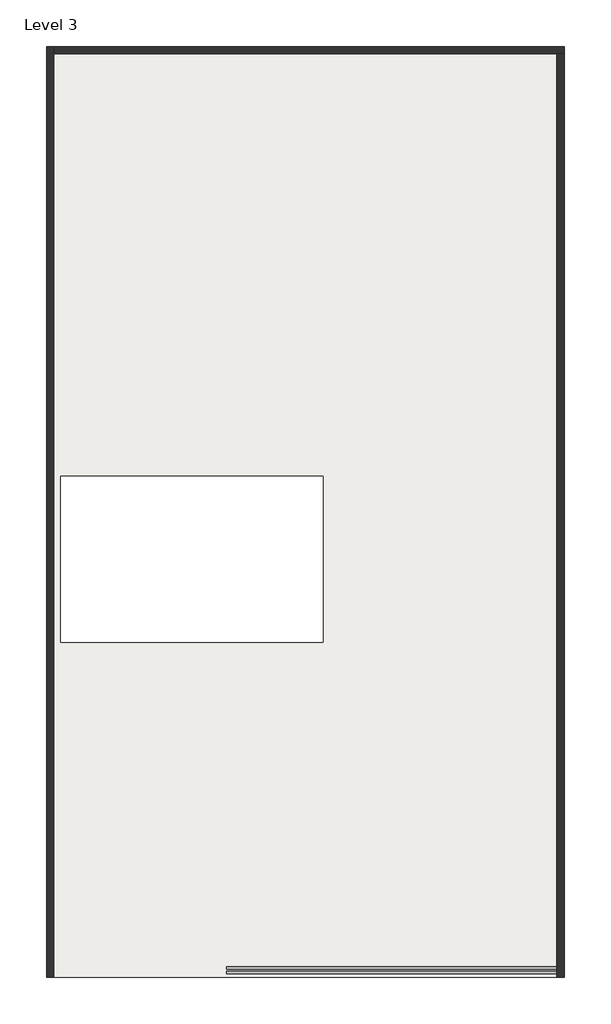
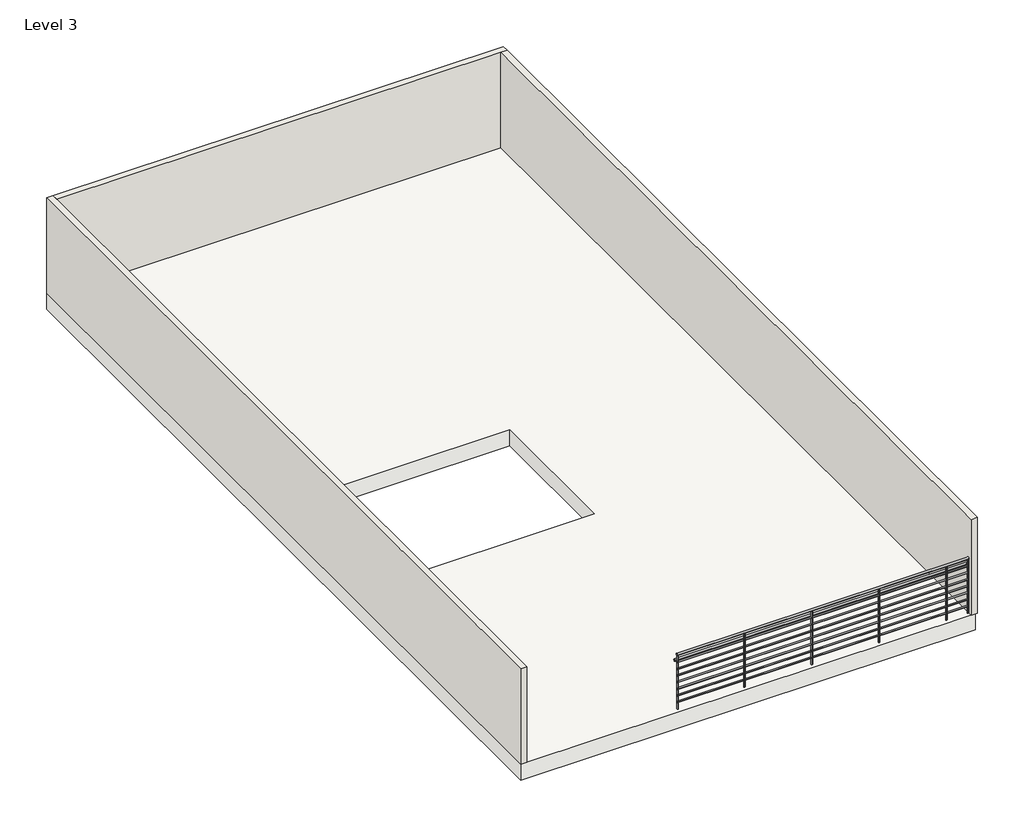
# One storey: 3 walls, 1 railing, 1 slab.
"""IFC4 building model written with IfcOpenShell, lengths in millimetres."""

from ifc_helpers import new_model, si_unit, point, frame, frame_2d, origin, place, context, project, spatial, polyline, circle_curve, trimmed, segment, composite_curve, outline, extrude, faceted_brep, element, save

model = new_model("IFC4")

# Units and contexts
model_context = context("Model", 3, world=origin())
ifc_project = project(units=[si_unit("LENGTHUNIT", "METRE", prefix="MILLI")], contexts=[model_context])

# Site, building, storey
site = spatial("IfcSite", under=ifc_project)
building = spatial("IfcBuilding", under=site)
storey = spatial("IfcBuildingStorey", under=building, Name="Level 3", Elevation=6400.8)

# Railing
placement = place(None, origin())
element("IfcRailing", 1, ObjectType="Guardrail - Pipe", at=placement, inside=storey, context=model_context, shape_type="SweptSolid", body=[
    extrude(outline(composite_curve([segment(trimmed(circle_curve(frame_2d((-4166.2834906, 7296.15)), 19.05), [point((-4185.3334906, 7296.15))], [point((-4147.2334906, 7296.15))], False, "CARTESIAN"), True, "CONTINUOUS"), segment(trimmed(circle_curve(frame_2d((-4166.2834906, 7296.15)), 19.05), [point((-4147.2334906, 7296.15))], [point((-4185.3334906, 7296.15))], False, "CARTESIAN"), True, "CONTINUOUS")], self_intersect=False)), frame((-11047.3280281, 0.0, 0.0), z_axis=(1.0, 0.0, 0.0), x_axis=(0.0, 1.0, 0.0)), (0.0, 0.0, 1.0), 5278.8112572),
    extrude(outline(composite_curve([segment(trimmed(circle_curve(frame_2d((-4242.4834906, 7448.55)), 19.05), [point((-4261.5334906, 7448.55))], [point((-4223.4334906, 7448.55))], False, "CARTESIAN"), True, "CONTINUOUS"), segment(trimmed(circle_curve(frame_2d((-4242.4834906, 7448.55)), 19.05), [point((-4223.4334906, 7448.55))], [point((-4261.5334906, 7448.55))], False, "CARTESIAN"), True, "CONTINUOUS")], self_intersect=False)), frame((-11047.3280281, 0.0, 0.0), z_axis=(1.0, 0.0, 0.0), x_axis=(0.0, 1.0, 0.0)), (0.0, 0.0, 1.0), 5278.8112572),
    extrude(outline(composite_curve([segment(trimmed(circle_curve(frame_2d((-4242.4834906, 7302.5)), 12.7), [point((-4229.7834906, 7302.5))], [point((-4255.1834906, 7302.5))], False, "CARTESIAN"), True, "CONTINUOUS"), segment(trimmed(circle_curve(frame_2d((-4242.4834906, 7302.5)), 12.7), [point((-4255.1834906, 7302.5))], [point((-4229.7834906, 7302.5))], False, "CARTESIAN"), True, "CONTINUOUS")], self_intersect=False)), frame((-11047.3280281, 0.0, 0.0), z_axis=(1.0, 0.0, 0.0), x_axis=(0.0, 1.0, 0.0)), (0.0, 0.0, 1.0), 5278.8112572),
    extrude(outline(composite_curve([segment(trimmed(circle_curve(frame_2d((-4242.4834906, 7175.5)), 12.7), [point((-4229.7834906, 7175.5))], [point((-4255.1834906, 7175.5))], False, "CARTESIAN"), True, "CONTINUOUS"), segment(trimmed(circle_curve(frame_2d((-4242.4834906, 7175.5)), 12.7), [point((-4255.1834906, 7175.5))], [point((-4229.7834906, 7175.5))], False, "CARTESIAN"), True, "CONTINUOUS")], self_intersect=False)), frame((-11047.3280281, 0.0, 0.0), z_axis=(1.0, 0.0, 0.0), x_axis=(0.0, 1.0, 0.0)), (0.0, 0.0, 1.0), 5278.8112572),
    extrude(outline(composite_curve([segment(trimmed(circle_curve(frame_2d((-4242.4834906, 7048.5)), 12.7), [point((-4229.7834906, 7048.5))], [point((-4255.1834906, 7048.5))], False, "CARTESIAN"), True, "CONTINUOUS"), segment(trimmed(circle_curve(frame_2d((-4242.4834906, 7048.5)), 12.7), [point((-4255.1834906, 7048.5))], [point((-4229.7834906, 7048.5))], False, "CARTESIAN"), True, "CONTINUOUS")], self_intersect=False)), frame((-11047.3280281, 0.0, 0.0), z_axis=(1.0, 0.0, 0.0), x_axis=(0.0, 1.0, 0.0)), (0.0, 0.0, 1.0), 5278.8112572),
    extrude(outline(composite_curve([segment(trimmed(circle_curve(frame_2d((-4242.4834906, 6921.5)), 12.7), [point((-4229.7834906, 6921.5))], [point((-4255.1834906, 6921.5))], False, "CARTESIAN"), True, "CONTINUOUS"), segment(trimmed(circle_curve(frame_2d((-4242.4834906, 6921.5)), 12.7), [point((-4255.1834906, 6921.5))], [point((-4229.7834906, 6921.5))], False, "CARTESIAN"), True, "CONTINUOUS")], self_intersect=False)), frame((-11047.3280281, 0.0, 0.0), z_axis=(1.0, 0.0, 0.0), x_axis=(0.0, 1.0, 0.0)), (0.0, 0.0, 1.0), 5278.8112572),
    extrude(outline(composite_curve([segment(trimmed(circle_curve(frame_2d((-4242.4834906, 6794.5)), 12.7), [point((-4229.7834906, 6794.5))], [point((-4255.1834906, 6794.5))], False, "CARTESIAN"), True, "CONTINUOUS"), segment(trimmed(circle_curve(frame_2d((-4242.4834906, 6794.5)), 12.7), [point((-4255.1834906, 6794.5))], [point((-4229.7834906, 6794.5))], False, "CARTESIAN"), True, "CONTINUOUS")], self_intersect=False)), frame((-11047.3280281, 0.0, 0.0), z_axis=(1.0, 0.0, 0.0), x_axis=(0.0, 1.0, 0.0)), (0.0, 0.0, 1.0), 5278.8112572),
    extrude(outline(composite_curve([segment(trimmed(circle_curve(frame_2d((-4242.4834906, 6667.5)), 12.7), [point((-4229.7834906, 6667.5))], [point((-4255.1834906, 6667.5))], False, "CARTESIAN"), True, "CONTINUOUS"), segment(trimmed(circle_curve(frame_2d((-4242.4834906, 6667.5)), 12.7), [point((-4255.1834906, 6667.5))], [point((-4229.7834906, 6667.5))], False, "CARTESIAN"), True, "CONTINUOUS")], self_intersect=False)), frame((-11047.3280281, 0.0, 0.0), z_axis=(1.0, 0.0, 0.0), x_axis=(0.0, 1.0, 0.0)), (0.0, 0.0, 1.0), 5278.8112572),
    extrude(outline(composite_curve([segment(trimmed(circle_curve(frame_2d((-4242.4834906, 6540.5)), 12.7), [point((-4229.7834906, 6540.5))], [point((-4255.1834906, 6540.5))], False, "CARTESIAN"), True, "CONTINUOUS"), segment(trimmed(circle_curve(frame_2d((-4242.4834906, 6540.5)), 12.7), [point((-4255.1834906, 6540.5))], [point((-4229.7834906, 6540.5))], False, "CARTESIAN"), True, "CONTINUOUS")], self_intersect=False)), frame((-11047.3280281, 0.0, 0.0), z_axis=(1.0, 0.0, 0.0), x_axis=(0.0, 1.0, 0.0)), (0.0, 0.0, 1.0), 5278.8112572),
    extrude(outline(composite_curve([segment(trimmed(circle_curve(frame_2d((-6170.5280281, -4242.4834906)), 12.7), [point((-6170.5280281, -4229.7834906))], [point((-6170.5280281, -4255.1834906))], False, "CARTESIAN"), True, "CONTINUOUS"), segment(trimmed(circle_curve(frame_2d((-6170.5280281, -4242.4834906)), 12.7), [point((-6170.5280281, -4255.1834906))], [point((-6170.5280281, -4229.7834906))], False, "CARTESIAN"), True, "CONTINUOUS")], self_intersect=False)), frame((0.0, 0.0, 6400.8), z_axis=(0.0, 0.0, 1.0), x_axis=(1.0, 0.0, 0.0)), (0.0, 0.0, 1.0), 1028.7),
    extrude(outline(composite_curve([segment(trimmed(circle_curve(frame_2d((-7389.7280281, -4242.4834906)), 12.7), [point((-7389.7280281, -4229.7834906))], [point((-7389.7280281, -4255.1834906))], False, "CARTESIAN"), True, "CONTINUOUS"), segment(trimmed(circle_curve(frame_2d((-7389.7280281, -4242.4834906)), 12.7), [point((-7389.7280281, -4255.1834906))], [point((-7389.7280281, -4229.7834906))], False, "CARTESIAN"), True, "CONTINUOUS")], self_intersect=False)), frame((0.0, 0.0, 6400.8), z_axis=(0.0, 0.0, 1.0), x_axis=(1.0, 0.0, 0.0)), (0.0, 0.0, 1.0), 1028.7),
    extrude(outline(composite_curve([segment(trimmed(circle_curve(frame_2d((-8608.9280281, -4242.4834906)), 12.7), [point((-8608.9280281, -4229.7834906))], [point((-8608.9280281, -4255.1834906))], False, "CARTESIAN"), True, "CONTINUOUS"), segment(trimmed(circle_curve(frame_2d((-8608.9280281, -4242.4834906)), 12.7), [point((-8608.9280281, -4255.1834906))], [point((-8608.9280281, -4229.7834906))], False, "CARTESIAN"), True, "CONTINUOUS")], self_intersect=False)), frame((0.0, 0.0, 6400.8), z_axis=(0.0, 0.0, 1.0), x_axis=(1.0, 0.0, 0.0)), (0.0, 0.0, 1.0), 1028.7),
    extrude(outline(composite_curve([segment(trimmed(circle_curve(frame_2d((-9828.1280281, -4242.4834906)), 12.7), [point((-9828.1280281, -4229.7834906))], [point((-9828.1280281, -4255.1834906))], False, "CARTESIAN"), True, "CONTINUOUS"), segment(trimmed(circle_curve(frame_2d((-9828.1280281, -4242.4834906)), 12.7), [point((-9828.1280281, -4255.1834906))], [point((-9828.1280281, -4229.7834906))], False, "CARTESIAN"), True, "CONTINUOUS")], self_intersect=False)), frame((0.0, 0.0, 6400.8), z_axis=(0.0, 0.0, 1.0), x_axis=(1.0, 0.0, 0.0)), (0.0, 0.0, 1.0), 1028.7),
    extrude(outline(composite_curve([segment(trimmed(circle_curve(frame_2d((-5781.2167709, -4242.4834906)), 12.7), [point((-5781.2167709, -4229.7834906))], [point((-5781.2167709, -4255.1834906))], False, "CARTESIAN"), True, "CONTINUOUS"), segment(trimmed(circle_curve(frame_2d((-5781.2167709, -4242.4834906)), 12.7), [point((-5781.2167709, -4255.1834906))], [point((-5781.2167709, -4229.7834906))], False, "CARTESIAN"), True, "CONTINUOUS")], self_intersect=False)), frame((0.0, 0.0, 6400.8), z_axis=(0.0, 0.0, 1.0), x_axis=(1.0, 0.0, 0.0)), (0.0, 0.0, 1.0), 1028.7),
    extrude(outline(composite_curve([segment(trimmed(circle_curve(frame_2d((-11034.6280281, -4242.4834906)), 12.7), [point((-11034.6280281, -4229.7834906))], [point((-11034.6280281, -4255.1834906))], False, "CARTESIAN"), True, "CONTINUOUS"), segment(trimmed(circle_curve(frame_2d((-11034.6280281, -4242.4834906)), 12.7), [point((-11034.6280281, -4255.1834906))], [point((-11034.6280281, -4229.7834906))], False, "CARTESIAN"), True, "CONTINUOUS")], self_intersect=False)), frame((0.0, 0.0, 6400.8), z_axis=(0.0, 0.0, 1.0), x_axis=(1.0, 0.0, 0.0)), (0.0, 0.0, 1.0), 1028.7),
])

# Slab
element("IfcSlab", 2, ObjectType="Generic - 12\"", at=placement, inside=storey, context=model_context, shape_type="SweptSolid", body=[
    extrude(outline(polyline([(-5692.3167709, 10539.0362133), (-5692.3167709, -4319.9637867), (-13921.9167709, -4319.9637867), (-13921.9167709, 10539.0362133), (-5692.3167709, 10539.0362133)]), holes=[polyline([(-9502.3167709, 3681.0362133), (-13693.3167709, 3681.0362133), (-13693.3167709, 1031.225127), (-9502.3167709, 1031.225127), (-9502.3167709, 3681.0362133)])]), frame((0.0, 0.0, 6096.0), z_axis=(0.0, 0.0, 1.0), x_axis=(1.0, 0.0, 0.0)), (0.0, 0.0, 1.0), 304.8),
])

# Walls
element("IfcWall", 3, ObjectType="4.5\" inner wall", at=placement, inside=storey, context=model_context, shape_type="Brep", body=[
    faceted_brep([(-13807.6167709, 10424.7362133, 6400.8), (-5768.5167709, 10424.7362133, 6400.8), (-5654.2167709, 10424.7362133, 6400.8), (-5654.2167709, 10424.7362133, 8229.6), (-5768.5167709, 10424.7362133, 8229.6), (-13807.6167709, 10424.7362133, 8229.6), (-13807.6167709, 10539.0362133, 6400.8), (-13807.6167709, 10539.0362133, 8229.6), (-5654.2167709, 10539.0362133, 8229.6), (-5654.2167709, 10539.0362133, 6400.8)], [[[0, 1, 2, 3, 4, 5]], [[6, 7, 8, 9]], [[2, 1, 0, 6, 9]], [[5, 4, 3, 8, 7]], [[3, 2, 9, 8]], [[0, 5, 7, 6]]]),
])
element("IfcWall", 4, ObjectType="4.5\" inner wall", at=placement, inside=storey, context=model_context, shape_type="SweptSolid", body=[
    extrude(outline(polyline([(-5768.5167709, -4319.9637867), (-5768.5167709, 10424.7362133), (-5654.2167709, 10424.7362133), (-5654.2167709, -4319.9637867), (-5768.5167709, -4319.9637867)])), frame((0.0, 0.0, 6400.8), z_axis=(0.0, 0.0, 1.0), x_axis=(1.0, 0.0, 0.0)), (0.0, 0.0, 1.0), 1828.8),
])
element("IfcWall", 5, ObjectType="4.5\" inner wall", at=placement, inside=storey, context=model_context, shape_type="Brep", body=[
    faceted_brep([(-13807.6167709, -4319.9637867, 6400.8), (-13807.6167709, 10424.7362133, 6400.8), (-13807.6167709, 10539.0362133, 6400.8), (-13807.6167709, 10539.0362133, 8229.6), (-13807.6167709, 10424.7362133, 8229.6), (-13807.6167709, -4319.9637867, 8229.6), (-13921.9167709, -4319.9637867, 6400.8), (-13921.9167709, -4319.9637867, 8229.6), (-13921.9167709, 10539.0362133, 8229.6), (-13921.9167709, 10539.0362133, 6400.8)], [[[0, 1, 2, 3, 4, 5]], [[6, 7, 8, 9]], [[2, 1, 0, 6, 9]], [[5, 4, 3, 8, 7]], [[0, 5, 7, 6]], [[3, 2, 9, 8]]]),
])

save(model, "model.ifc")

# Revit data of these elements
# Type "Guardrail - Pipe"
#   Assembly Code = "C2010400"
#   built-in parameter 1008612 = 0.0416667 (stored number, unit not read)
#   built-in parameter 1008611 = 0.0833333 (stored number, unit not read)
#   built-in parameter 1008609 = 4 (stored number, unit not read)
#   built-in parameter 1008604 = 0.166667 (stored number, unit not read)
#   built-in parameter 1008603 = 0.166667 (stored number, unit not read)
#   Railing Height = 3' - 6"
#   built-in parameter 1008630 = 2
#   built-in parameter 1008610 = 1
#   built-in parameter 1008605 = 1
#   built-in parameter 1008618 = Baluster - Round : 1"
# Type "Generic - 12\""
#   Assembly Code = "B1010"
#   Function = 0
#   Layers, outside or top first: 1' - 0" no material (function 1)
# Type "4.5\" inner wall"
#   Assembly Code = "B2010"
#   Layers, outside or top first: 0' - 4 1/2" no material (function 1)
# Element 1 (IfcRailing, "Guardrail - Pipe")
#   Phase Created = New Construction
# Element 2 (IfcSlab, "Generic - 12\"")
#   Height Offset From Level = 0' - 0"
#   Phase Created = New Construction
#   Materials on its faces: "Default Floor"
# Elements 3, 4, 5 (IfcWall, "4.5\" inner wall")
#   Top Offset = 0' - 0"
#   Base Offset = 0' - 0"
#   Unconnected Height = 6' - 0"
#   wall height = 6' - 0"
#   Phase Created = New Construction
#   Base Constraint = Level 3
#   Materials on its faces: "Default Wall"
# Materials
#   "Default Floor": colour RGB 128 128 128, transparency 0, Cost = 0
#   "Default Wall": colour RGB 128 128 128, transparency 0, Cost = 0
